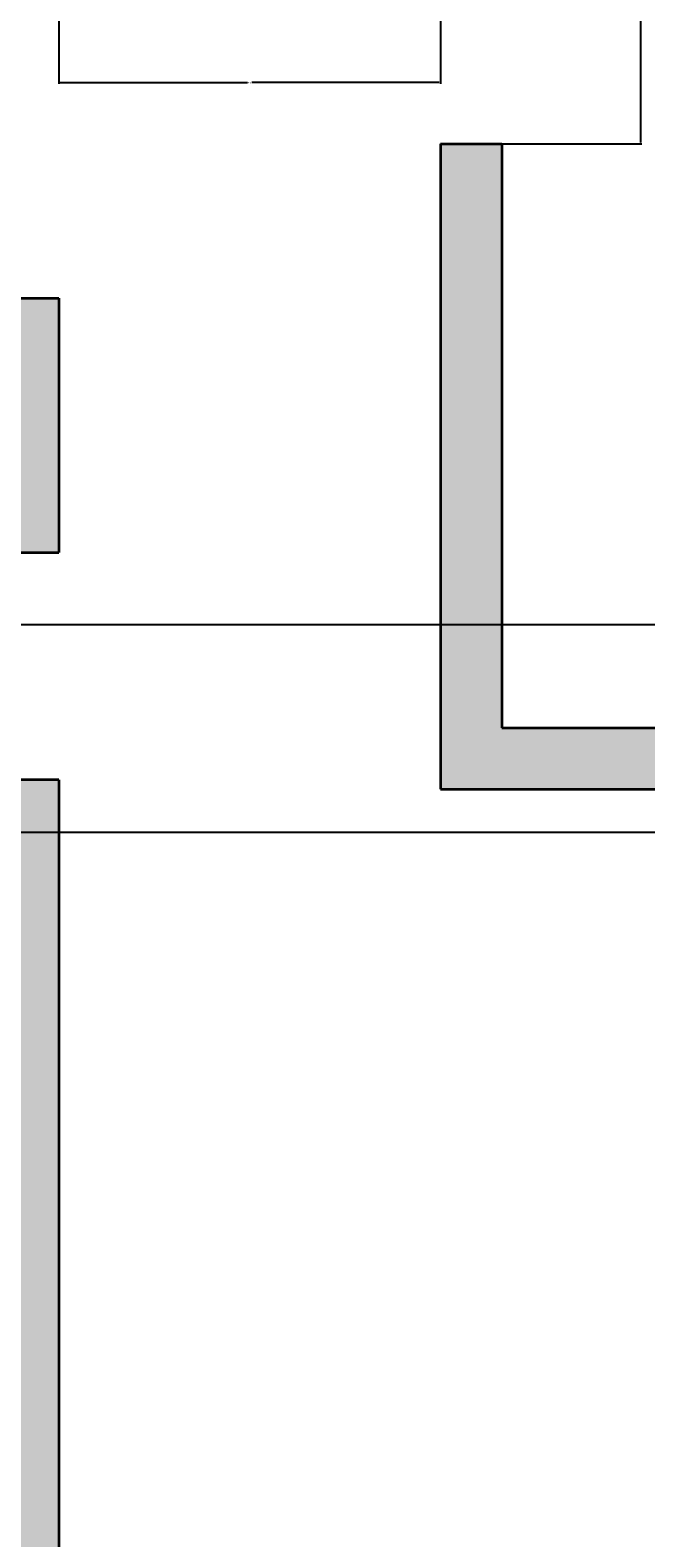
# Model space of a CAD drawing. Units: inches. Extents: x 0 to 423, y -517 to 94.
# Tile 3 of 8: x 182 to 273, y -382 to -160. Entities that reach past the tile are written whole.
import ezdxf

# ---------------------------------------------------------------- set-up
doc = ezdxf.new("R2010")
doc.units = ezdxf.units.IN
doc.header["$MEASUREMENT"] = 0
doc.layers.add('A-ANNO-DIMS', color=2, linetype='Continuous', lineweight=18)
doc.layers.add('A-WALL', color=7, linetype='Continuous', lineweight=35)
doc.layers.add('A-WALL-PATT', color=30, linetype='Continuous', lineweight=13, true_color=0xf26722)
doc.styles.get("Standard").update_dxf_attribs({"font": 'arial.ttf'})
doc.dimstyles.get("Standard").update_dxf_attribs({"dimtxt": 0.18, "dimasz": 0.18, "dimexe": 0.18, "dimexo": 0.0625, "dimgap": 0.09, "dimtad": 0, "dimtih": 1, "dimtoh": 1, "dimdec": 0, "dimzin": 0, "dimdsep": 46, "dimlunit": 3, "dimtxsty": 'Standard', "dimcen": 0.09, "dimadec": 0, "dimazin": 0, "dimtfac": 1, "dimtdec": 0, "dimtofl": 0, "dimtmove": 0, "dimatfit": 3, "dimfxl": 1, "dimtolj": 1, "dimtzin": 0, "dimarcsym": 0})

# ---------------------------------------------------------------- blocks, each defined once
blk = doc.blocks.new('*D53')
at = {"layer": 'A-ANNO-DIMS', "color": 0, "lineweight": -2, "transparency": 16777216}
for p, q in [((85.83, -247.61), (422.3, -247.61)), ((422.12, -247.79), (422.12, -262.66)), ((422.12, -277.89), (422.12, -263.02)), ((80.68, -278.07), (422.3, -278.07))]:
    blk.add_line(p, q, dxfattribs=at)
at = {"layer": 'A-ANNO-DIMS', "color": 0, "transparency": 16777216}
for points in [[(422.09, -247.79), (422.15, -247.79), (422.12, -247.61)], [(422.09, -277.89), (422.15, -277.89), (422.12, -278.07)]]:
    blk.add_solid(points, dxfattribs=at)
at = {"layer": 'Defpoints', "color": 0, "transparency": 16777216}
for p in [(85.77, -247.61), (80.61, -278.07), (422.12, -278.07)]:
    blk.add_point(p, dxfattribs=at)
at = {"layer": 'A-ANNO-DIMS', "color": 0, "transparency": 16777216, "insert": (422.12, -262.84), "char_height": 0.18, "attachment_point": 5}
blk.add_mtext('\\A1;2\'-6 1/2"', dxfattribs=at)
blk = doc.blocks.new('*D55')
at = {"layer": 'A-ANNO-DIMS', "color": 0, "lineweight": -2, "transparency": 16777216}
for p, q in [((242.79, -138.77), (272.3, -138.77)), ((272.12, -138.95), (272.12, -157.77)), ((272.12, -176.96), (272.12, -158.14)), ((242.79, -177.14), (272.3, -177.14))]:
    blk.add_line(p, q, dxfattribs=at)
at = {"layer": 'A-ANNO-DIMS', "color": 0, "transparency": 16777216}
for points in [[(272.09, -138.95), (272.15, -138.95), (272.12, -138.77)], [(272.09, -176.96), (272.15, -176.96), (272.12, -177.14)]]:
    blk.add_solid(points, dxfattribs=at)
at = {"layer": 'Defpoints', "color": 0, "transparency": 16777216}
for p in [(242.72, -138.77), (242.72, -177.14), (272.12, -177.14)]:
    blk.add_point(p, dxfattribs=at)
at = {"layer": 'A-ANNO-DIMS', "color": 0, "transparency": 16777216, "insert": (272.12, -157.95), "char_height": 0.18, "attachment_point": 5}
blk.add_mtext('\\A1;3\'-2 1/2"', dxfattribs=at)
blk = doc.blocks.new('*D65')
at = {"layer": 'A-ANNO-DIMS', "color": 0, "lineweight": -2, "transparency": 16777216}
for p, q in [((186.72, -138.83), (186.72, -168.35)), ((242.72, -138.83), (242.72, -168.35)), ((186.9, -168.17), (214.39, -168.17)), ((242.54, -168.17), (215.06, -168.17))]:
    blk.add_line(p, q, dxfattribs=at)
at = {"layer": 'A-ANNO-DIMS', "color": 0, "transparency": 16777216}
for points in [[(186.9, -168.14), (186.9, -168.2), (186.72, -168.17)], [(242.54, -168.14), (242.54, -168.2), (242.72, -168.17)]]:
    blk.add_solid(points, dxfattribs=at)
at = {"layer": 'Defpoints', "color": 0, "transparency": 16777216}
for p in [(186.72, -138.77), (242.72, -138.77), (186.72, -168.17)]:
    blk.add_point(p, dxfattribs=at)
at = {"layer": 'A-ANNO-DIMS', "color": 0, "transparency": 16777216, "insert": (214.72, -168.17), "char_height": 0.18, "attachment_point": 5}
blk.add_mtext('\\A1;4\'-8"', dxfattribs=at)

msp = doc.modelspace()

# ---------------------------------------------------------------- hatches: boundary and pattern name
at = {"layer": 'A-WALL-PATT'}
h = msp.add_hatch(color=256, dxfattribs=at)
h.dxf.hatch_style = 1
h.paths.add_polyline_path([(201.52, 16.23), (138.22, 16.23), (138.22, 7.23), (177.72, 7.23), (177.72, -138.77), (186.72, -138.77), (186.72, -92.77), (251.72, -92.77), (251.72, -22.53), (242.72, -22.53), (242.72, -83.77), (186.72, -83.77), (186.72, 7.23), (201.52, 7.23)])
h.paths.add_polyline_path([(78.22, 16.23), (29.72, 16.23), (29.72, -31.27), (38.72, -31.27), (38.72, 7.23), (78.22, 7.23)])
h.paths.add_polyline_path([(275.31, 16.23), (225.52, 16.23), (225.52, 7.23), (275.31, 7.23)])
h.paths.add_polyline_path([(392.72, 16.23), (335.31, 16.23), (335.31, 7.23), (383.72, 7.23), (383.72, -31.27), (392.72, -31.27)])
h.paths.add_polyline_path([(143.33, -129.77), (38.72, -129.77), (38.72, -91.27), (29.72, -91.27), (29.72, -157.27), (38.72, -157.27), (38.72, -138.77), (143.33, -138.77)])
h.paths.add_polyline_path([(186.72, -199.77), (38.72, -199.77), (38.72, -181.27), (29.72, -181.27), (29.72, -239.27), (38.72, -239.27), (38.72, -208.77), (177.72, -208.77), (177.72, -237.07), (186.72, -237.07)])
h.paths.add_polyline_path([(111.72, -161.55), (102.72, -161.55), (102.72, -199.77), (111.72, -199.77)])
h.paths.add_polyline_path([(392.72, -91.27), (383.72, -91.27), (383.72, -129.77), (242.72, -129.77), (242.72, -138.77), (383.72, -138.77), (383.72, -169.77), (392.72, -169.77)])
h.paths.add_polyline_path([(392.72, -229.77), (383.72, -229.77), (383.72, -262.77), (251.72, -262.77), (251.72, -177.14), (242.72, -177.14), (242.72, -271.77), (383.72, -271.77), (383.72, -300.77), (392.72, -300.77)])
h.paths.add_polyline_path([(392.72, -360.77), (383.72, -360.77), (383.72, -389.77), (378.42, -389.77), (378.42, -398.77), (383.72, -398.77), (383.72, -458.77), (382.72, -458.77), (382.72, -467.77), (392.72, -467.77)])
h.paths.add_polyline_path([(364.92, -389.77), (348.72, -389.77), (348.72, -467.77), (358.72, -467.77), (358.72, -458.77), (357.72, -458.77), (357.72, -398.77), (364.92, -398.77)])
h.paths.add_polyline_path([(320.72, -389.77), (283.72, -389.77), (283.72, -398.77), (320.72, -398.77)])
h.paths.add_polyline_path([(223.72, -389.77), (186.72, -389.77), (186.72, -270.38), (177.72, -270.38), (177.72, -458.77), (138.22, -458.77), (138.22, -467.77), (186.72, -467.77), (186.72, -398.77), (223.72, -398.77)])
h.paths.add_polyline_path([(143.29, -329.77), (38.72, -329.77), (38.72, -299.27), (29.72, -299.27), (29.72, -338.77), (143.29, -338.77)])
h.paths.add_polyline_path([(38.72, -374.71), (29.72, -374.71), (29.72, -398.74), (38.72, -398.74)])
h.paths.add_polyline_path([(78.22, -458.77), (38.72, -458.77), (38.72, -434.74), (29.72, -434.74), (29.72, -467.77), (78.22, -467.77)])
h.paths.add_polyline_path([(279.99, -158.17), (326.6, -158.17), (326.6, -135.78), (279.99, -135.78)], flags=25)
h.paths.add_polyline_path([(355.56, -439.13), (387, -439.13), (387, -416.66), (355.56, -416.66)], flags=9)

# ---------------------------------------------------------------- linework, layer by layer
at = {"layer": 'A-WALL'}
for p, q in [((242.72, -177.14), (251.72, -177.14)), ((242.72, -177.14), (242.72, -271.77)), ((251.72, -177.14), (251.72, -262.77)), ((38.72, -199.77), (186.72, -199.77)), ((186.72, -199.77), (186.72, -237.07)), ((177.72, -237.07), (186.72, -237.07)), ((251.72, -262.77), (383.72, -262.77)), ((186.72, -270.38), (177.72, -270.38)), ((186.72, -270.38), (186.72, -389.77)), ((242.72, -271.77), (383.72, -271.77))]:
    msp.add_line(p, q, dxfattribs=at)

# ---------------------------------------------------------------- dimensions: what is measured, and where the dimension line sits
at = {"layer": 'A-ANNO-DIMS'}
for base, p1, p2, angle, picture, middle in [((186.72, -168.17), (242.72, -138.77), (186.72, -138.77), 180, '*D65', (214.72, -168.17)), ((272.12, -177.14), (242.72, -138.77), (242.72, -177.14), 270, '*D55', (272.12, -157.95)), ((422.12, -278.07), (85.77, -247.61), (80.61, -278.07), 90, '*D53', (422.12, -262.84))]:
    dim = msp.add_linear_dim(base=base, p1=p1, p2=p2, angle=angle, dimstyle='Standard', override={"dimdec": 1, "dimlfac": 1, "dimrnd": 0, "dimzin": 1, "dimdsep": 46, "dimlunit": 4, "dimfrac": 2}, dxfattribs=at)
    dim.commit()
    dim.dimension.update_dxf_attribs({"geometry": picture, "text_midpoint": middle})

doc.saveas('drawing.dxf')
